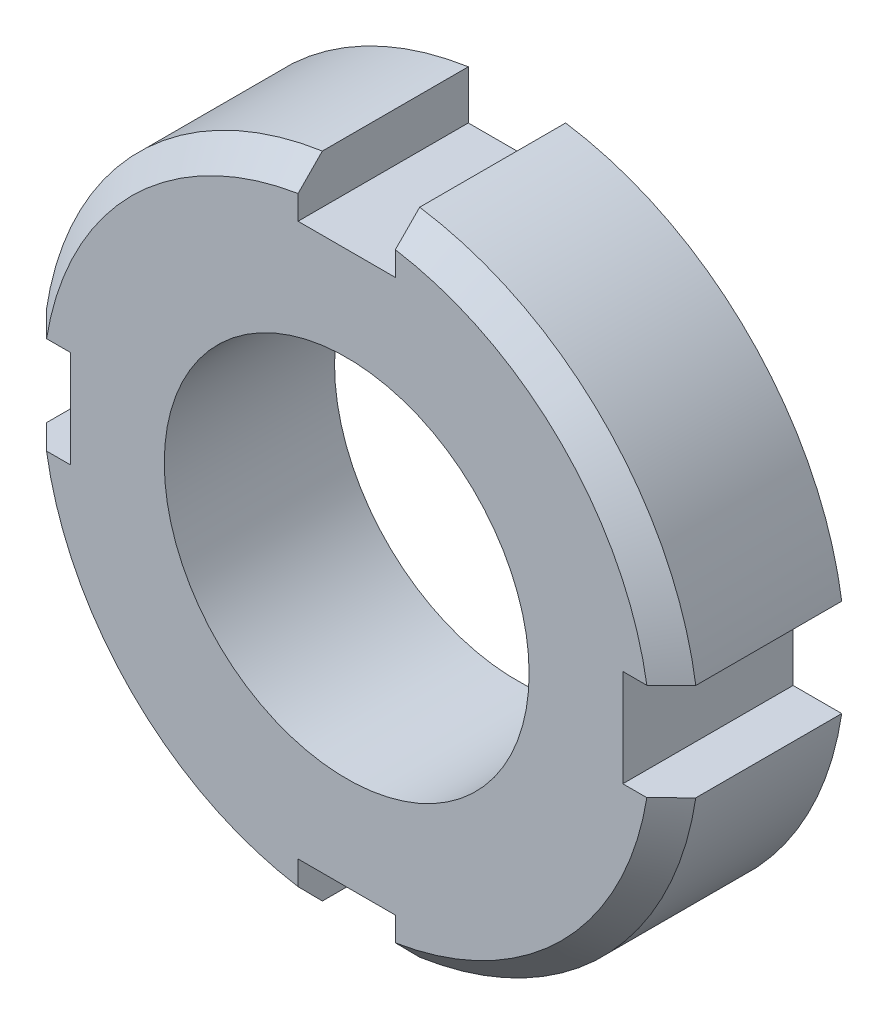
SolidWorks part; units mm, degrees
material "Plain Carbon Steel"
ref_plane "Front Plane" through (0, 0, 0) normal (0, 0, 1) x (1, 0, 0)
ref_plane "Top Plane" through (0, 0, 0) normal (0, 1, 0) x (1, 0, 0)
ref_plane "Right Plane" through (0, 0, 0) normal (1, 0, 0) x (0, 0, -1)
sketch "Slotted Nut Profile Ø27" plane through (0, 0, 0) normal (0, 0, 1) x (1, 0, 0)
  line L0 (0, 0) -> (0, 13.5) construction
  line L1 (2, 11.351) -> (2, 13.351)
  line L2 (-2, 11.351) -> (-2, 13.351)
  line L3 (-2, 11.351) -> (2, 11.351)
  line L4 (11.351, 2) -> (13.351, 2)
  line L5 (-2, 0) -> (-2, 13.5) construction
  line L6 (2, 0) -> (2, 13.5) construction
  line L7 (11.351, 2) -> (11.351, -2)
  line L8 (11.351, -2) -> (13.351, -2)
  line L9 (2, -11.351) -> (2, -13.351)
  line L10 (2, -11.351) -> (-2, -11.351)
  line L11 (-2, -11.351) -> (-2, -13.351)
  line L12 (-11.351, -2) -> (-13.351, -2)
  line L13 (-11.351, -2) -> (-11.351, 2)
  line L14 (-11.351, 2) -> (-13.351, 2)
  arc A0 (-2, 13.351) -> (-13.351, 2) centre (0, 0) ccw
  arc A1 (-13.351, -2) -> (-2, -13.351) centre (0, 0) ccw
  arc A2 (2, -13.351) -> (13.351, -2) centre (0, 0) ccw
  arc A3 (13.351, 2) -> (2, 13.351) centre (0, 0) ccw
  point P26 (0, 0)
  dimension "D1" = 27
  dimension "D4" = 2
  dimension "D2" = 2
  dimension "D3" = 2
  dimension "D5" = 4
extrude "Nut Body 7mm" add sketch "Slotted Nut Profile Ø27" along normal mid plane 7
sketch "Bore Sketch Ø15" plane through (0, 0, 3.5) normal (0, 0, 1) x (1, 0, 0)
  circle A0 centre (0, 0) radius 7.5
  dimension "D1" = 15
extrude "Bore Ø15" cut sketch "Bore Sketch Ø15" against normal through all both
cosmetic thread "Cosmetic Thread1" parameters "D2"=18
cosmetic thread "Cosmetic Thread2" parameters "D2"=18
chamfer "Edge Chamfers 1x45°" distance 1 angle 45 4 edges at (9.5459, -9.5459, 3.5) (-9.5459, -9.5459, 3.5) (-9.5459, 9.5459, 3.5) (9.5459, 9.5459, 3.5)
